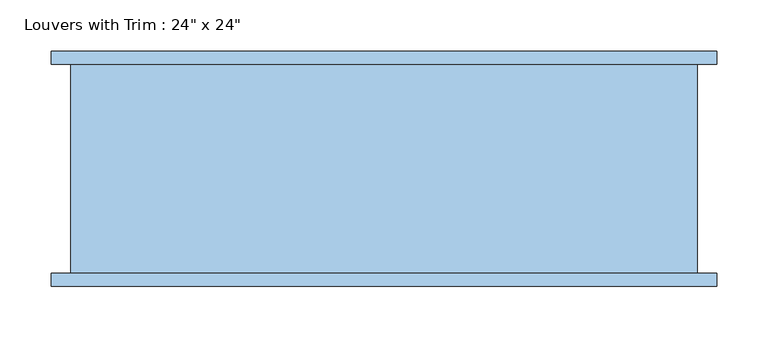
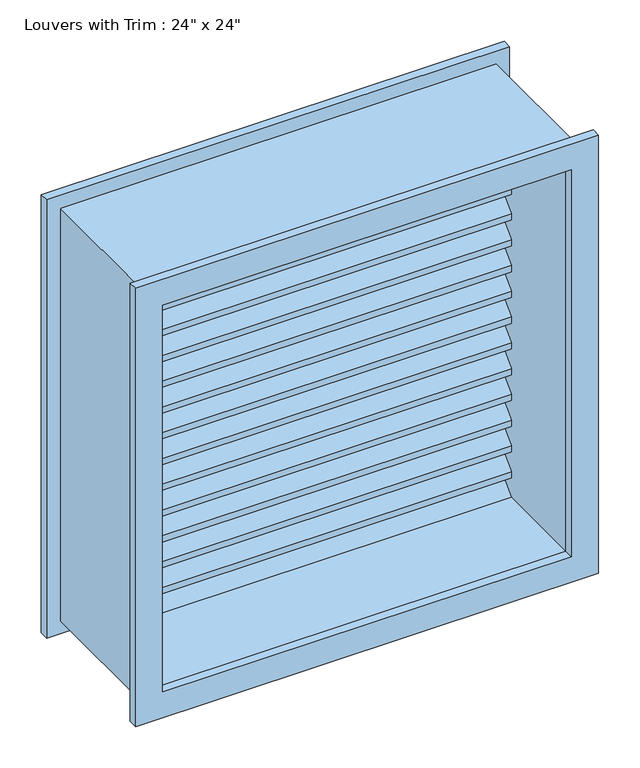
"""IFC4 building model written with IfcOpenShell, lengths in millimetres: window geometry."""

from ifc_helpers import new_model, si_unit, frame, origin, place, context, project, spatial, polyline, outline, extrude, source, transform, mapped, element, save


def window_0038ecf3(model_context):
    return source(origin(), model_context, "Body", "SweptSolid", [
        extrude(outline(polyline([(1543.05, -323.85), (895.35, -323.85), (895.35, 323.85), (1543.05, 323.85), (1543.05, -323.85)]), holes=[polyline([(1504.95, -285.75), (1504.95, 285.75), (933.45, 285.75), (933.45, -285.75), (1504.95, -285.75)])]), frame((0.0, 95.25, 0.0), z_axis=(0.0, 1.0, 0.0), x_axis=(0.0, 0.0, 1.0)), (0.0, 0.0, 1.0), 12.7),
        extrude(outline(polyline([(1543.05, 323.85), (1543.05, -323.85), (895.35, -323.85), (895.35, 323.85), (1543.05, 323.85)]), holes=[polyline([(1504.95, 285.75), (933.45, 285.75), (933.45, -285.75), (1504.95, -285.75), (1504.95, 285.75)])]), frame((0.0, -120.65, 0.0), z_axis=(0.0, 1.0, 0.0), x_axis=(0.0, 0.0, 1.0)), (0.0, 0.0, 1.0), 12.7),
        extrude(outline(polyline([(1524.0, 304.8), (1524.0, -304.8), (914.4, -304.8), (914.4, 304.8), (1524.0, 304.8)]), holes=[polyline([(1504.95, 285.75), (933.45, 285.75), (933.45, -285.75), (1504.95, -285.75), (1504.95, 285.75)])]), frame((0.0, -107.95, 0.0), z_axis=(0.0, 1.0, 0.0), x_axis=(0.0, 0.0, 1.0)), (0.0, 0.0, 1.0), 203.2),
        extrude(outline(polyline([(59.3289755, 969.3710245), (95.25, 933.45), (86.2697439, 933.45), (59.3289755, 960.3907684), (32.3882072, 933.45), (23.407951, 933.45), (59.3289755, 969.3710245)])), frame((-285.75, 0.0, 0.0), z_axis=(1.0, 0.0, 0.0), x_axis=(0.0, 1.0, 0.0)), (0.0, 0.0, 1.0), 571.5),
        extrude(outline(polyline([(59.3289755, 1007.4710245), (95.25, 971.55), (95.25, 962.5697439), (59.3289755, 998.4907684), (23.407951, 962.5697439), (23.407951, 971.55), (59.3289755, 1007.4710245)])), frame((-285.75, 0.0, 0.0), z_axis=(1.0, 0.0, 0.0), x_axis=(0.0, 1.0, 0.0)), (0.0, 0.0, 1.0), 571.5),
        extrude(outline(polyline([(59.3289755, 1045.5710245), (95.25, 1009.65), (95.25, 1000.6697439), (59.3289755, 1036.5907684), (23.407951, 1000.6697439), (23.407951, 1009.65), (59.3289755, 1045.5710245)])), frame((-285.75, 0.0, 0.0), z_axis=(1.0, 0.0, 0.0), x_axis=(0.0, 1.0, 0.0)), (0.0, 0.0, 1.0), 571.5),
        extrude(outline(polyline([(59.3289755, 1083.6710245), (95.25, 1047.75), (95.25, 1038.7697439), (59.3289755, 1074.6907684), (23.407951, 1038.7697439), (23.407951, 1047.75), (59.3289755, 1083.6710245)])), frame((-285.75, 0.0, 0.0), z_axis=(1.0, 0.0, 0.0), x_axis=(0.0, 1.0, 0.0)), (0.0, 0.0, 1.0), 571.5),
        extrude(outline(polyline([(59.3289755, 1121.7710245), (95.25, 1085.85), (95.25, 1076.8697439), (59.3289755, 1112.7907684), (23.407951, 1076.8697439), (23.407951, 1085.85), (59.3289755, 1121.7710245)])), frame((-285.75, 0.0, 0.0), z_axis=(1.0, 0.0, 0.0), x_axis=(0.0, 1.0, 0.0)), (0.0, 0.0, 1.0), 571.5),
        extrude(outline(polyline([(59.3289755, 1159.8710245), (95.25, 1123.95), (95.25, 1114.9697439), (59.3289755, 1150.8907684), (23.407951, 1114.9697439), (23.407951, 1123.95), (59.3289755, 1159.8710245)])), frame((-285.75, 0.0, 0.0), z_axis=(1.0, 0.0, 0.0), x_axis=(0.0, 1.0, 0.0)), (0.0, 0.0, 1.0), 571.5),
        extrude(outline(polyline([(59.3289755, 1197.9710245), (95.25, 1162.05), (95.25, 1153.0697439), (59.3289755, 1188.9907684), (23.407951, 1153.0697439), (23.407951, 1162.05), (59.3289755, 1197.9710245)])), frame((-285.75, 0.0, 0.0), z_axis=(1.0, 0.0, 0.0), x_axis=(0.0, 1.0, 0.0)), (0.0, 0.0, 1.0), 571.5),
        extrude(outline(polyline([(59.3289755, 1236.0710245), (95.25, 1200.15), (95.25, 1191.1697439), (59.3289755, 1227.0907684), (23.407951, 1191.1697439), (23.407951, 1200.15), (59.3289755, 1236.0710245)])), frame((-285.75, 0.0, 0.0), z_axis=(1.0, 0.0, 0.0), x_axis=(0.0, 1.0, 0.0)), (0.0, 0.0, 1.0), 571.5),
        extrude(outline(polyline([(59.3289755, 1274.1710245), (95.25, 1238.25), (95.25, 1229.2697439), (59.3289755, 1265.1907684), (23.407951, 1229.2697439), (23.407951, 1238.25), (59.3289755, 1274.1710245)])), frame((-285.75, 0.0, 0.0), z_axis=(1.0, 0.0, 0.0), x_axis=(0.0, 1.0, 0.0)), (0.0, 0.0, 1.0), 571.5),
        extrude(outline(polyline([(59.3289755, 1312.2710245), (95.25, 1276.35), (95.25, 1267.3697439), (59.3289755, 1303.2907684), (23.407951, 1267.3697439), (23.407951, 1276.35), (59.3289755, 1312.2710245)])), frame((-285.75, 0.0, 0.0), z_axis=(1.0, 0.0, 0.0), x_axis=(0.0, 1.0, 0.0)), (0.0, 0.0, 1.0), 571.5),
        extrude(outline(polyline([(59.3289755, 1350.3710245), (95.25, 1314.45), (95.25, 1305.4697439), (59.3289755, 1341.3907684), (23.407951, 1305.4697439), (23.407951, 1314.45), (59.3289755, 1350.3710245)])), frame((-285.75, 0.0, 0.0), z_axis=(1.0, 0.0, 0.0), x_axis=(0.0, 1.0, 0.0)), (0.0, 0.0, 1.0), 571.5),
        extrude(outline(polyline([(59.3289755, 1388.4710245), (95.25, 1352.55), (95.25, 1343.5697439), (59.3289755, 1379.4907684), (23.407951, 1343.5697439), (23.407951, 1352.55), (59.3289755, 1388.4710245)])), frame((-285.75, 0.0, 0.0), z_axis=(1.0, 0.0, 0.0), x_axis=(0.0, 1.0, 0.0)), (0.0, 0.0, 1.0), 571.5),
        extrude(outline(polyline([(59.3289755, 1426.5710245), (95.25, 1390.65), (95.25, 1381.6697439), (59.3289755, 1417.5907684), (23.407951, 1381.6697439), (23.407951, 1390.65), (59.3289755, 1426.5710245)])), frame((-285.75, 0.0, 0.0), z_axis=(1.0, 0.0, 0.0), x_axis=(0.0, 1.0, 0.0)), (0.0, 0.0, 1.0), 571.5),
        extrude(outline(polyline([(59.3289755, 1464.6710245), (95.25, 1428.75), (95.25, 1419.7697439), (59.3289755, 1455.6907684), (23.407951, 1419.7697439), (23.407951, 1428.75), (59.3289755, 1464.6710245)])), frame((-285.75, 0.0, 0.0), z_axis=(1.0, 0.0, 0.0), x_axis=(0.0, 1.0, 0.0)), (0.0, 0.0, 1.0), 571.5),
        extrude(outline(polyline([(59.3289755, 1502.7710245), (95.25, 1466.85), (95.25, 1457.8697439), (59.3289755, 1493.7907684), (23.407951, 1457.8697439), (23.407951, 1466.85), (59.3289755, 1502.7710245)])), frame((-285.75, 0.0, 0.0), z_axis=(1.0, 0.0, 0.0), x_axis=(0.0, 1.0, 0.0)), (0.0, 0.0, 1.0), 571.5),
    ])


if __name__ == "__main__":
    model = new_model("IFC4")
    model_context = context("Model", 3, world=origin())
    ifc_project = project(units=[si_unit("LENGTHUNIT", "METRE", prefix="MILLI")], contexts=[model_context])
    site = spatial("IfcSite", under=ifc_project)
    building = spatial("IfcBuilding", under=site)
    placement = place(None, origin())
    window_shape = window_0038ecf3(model_context)
    element("IfcWindow", 1, ObjectType="Louvers with Trim : 24\" x 24\"", at=placement, inside=building, context=model_context, shape_type="MappedRepresentation", body=[
        mapped(window_shape, transform((0.0, 0.0, 0.0), x_axis=(1.0, 0.0, 0.0), y_axis=(0.0, 1.0, 0.0), z_axis=(0.0, 0.0, 1.0))),
    ])
    save(model, "model.ifc")

# Revit data of these elements
# Type "Louvers with Trim : 24\" x 24\""
#   Type Mark = "27"
#   Construction Type Id = "GSP4R"
#   Assembly Code = "B20"
#   Analytic Construction = "1/8 in Pilkington single glazing"
#   Visual Light Transmittance = 0.9
#   Solar Heat Gain Coefficient = 0.78
#   Heat Transfer Coefficient (U) = 3.6886 W/(m²·K)
#   Default Sill Height = 3' - 0"
#   Trim Projection - Ext. = 0' - 0 1/2"
#   Trim Projection - Int. = 0' - 0 1/2"
#   Trim Width - Exterior = 0' - 1 1/2"
#   Trim Width - Interior = 0' - 1 1/2"
#   Width = 2' - 0"
#   Frame Material = Iron, Ductile
#   Louver Material = Glass
#   Trim Exterior Material = Glass
#   Trim Interior Material = Iron, Ductile
#   Wall Closure = (empty or 0)
# Element 1 (IfcWindow, "Louvers with Trim : 24\" x 24\"")
#   Materials on its faces: "Glass", "Iron, Ductile"
# Materials
#   "Iron, Ductile": class "Metal", colour RGB 0 0 0, transparency 0, Description = "Ductile cast iron", Cost = 0
#   "Glass": class "Glass", colour RGB 0 128 192, transparency 0.75, Description = "Soda Lime Glass", Cost = 0
